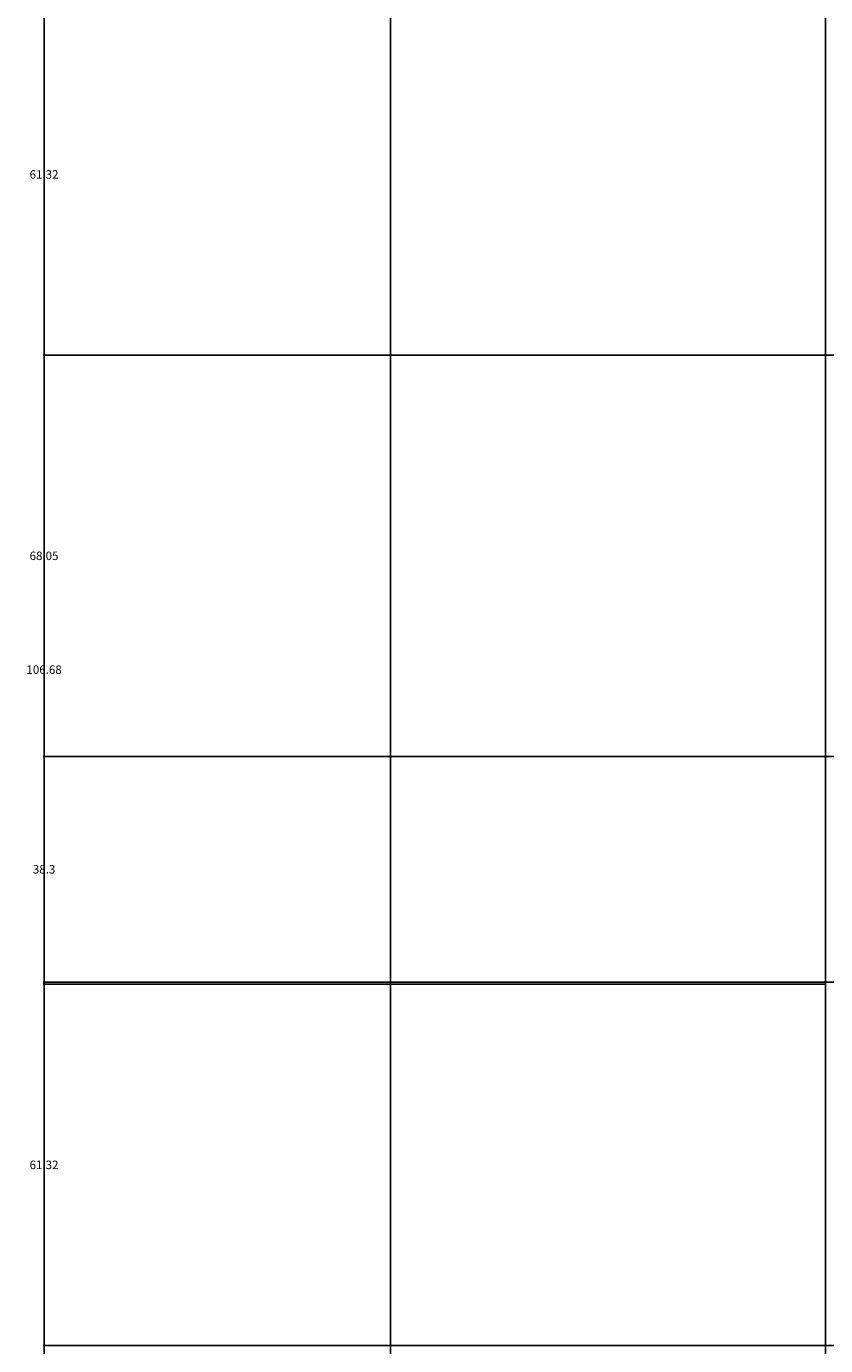
# Model space of a CAD drawing. Units: inches. Extents: x 241 to 943, y 109 to 1396.
# Tile 18 of 34: x 241 to 377, y 842 to 1065. Entities that reach past the tile are written whole.
import ezdxf

# ---------------------------------------------------------------- set-up
doc = ezdxf.new("R2010")
doc.units = ezdxf.units.IN
doc.header["$MEASUREMENT"] = 0
doc.layers.add('A-ANNO-DIMS', color=2, linetype='Continuous', lineweight=18)
doc.styles.get("Standard").update_dxf_attribs({"font": 'arial.ttf'})
doc.dimstyles.get("Standard").update_dxf_attribs({"dimtxt": 1.4375, "dimasz": 0.18, "dimexe": 0.18, "dimexo": 0.0625, "dimgap": 0.09, "dimtad": 0, "dimtih": 1, "dimtoh": 1, "dimdec": 4, "dimzin": 0, "dimdsep": 46, "dimlunit": 4, "dimtxsty": 'Standard', "dimcen": 0.09, "dimadec": 0, "dimazin": 0, "dimtfac": 1, "dimtdec": 4, "dimtofl": 0, "dimtmove": 0, "dimatfit": 3, "dimfxl": 1, "dimtolj": 1, "dimtzin": 0, "dimarcsym": 0})

# ---------------------------------------------------------------- blocks, each defined once
blk = doc.blocks.new('*D5')
at = {"layer": 'A-ANNO-DIMS', "color": 0, "lineweight": -2, "transparency": 16777216}
for p, q in [((303.24, 177.8), (303.24, 1395.05)), ((303.42, 1394.87), (338.18, 1394.87)), ((376.86, 1394.87), (342.09, 1394.87)), ((377.04, 177.76), (377.04, 1395.05))]:
    blk.add_line(p, q, dxfattribs=at)
at = {"layer": 'A-ANNO-DIMS', "color": 0, "transparency": 16777216}
for points in [[(303.42, 1394.9), (303.42, 1394.84), (303.24, 1394.87)], [(376.86, 1394.9), (376.86, 1394.84), (377.04, 1394.87)]]:
    blk.add_solid(points, dxfattribs=at)
at = {"layer": 'Defpoints', "color": 0, "transparency": 16777216}
for p in [(377.04, 1394.87), (303.24, 177.74), (377.04, 177.7)]:
    blk.add_point(p, dxfattribs=at)
at = {"layer": 'A-ANNO-DIMS', "color": 0, "transparency": 16777216, "insert": (340.14, 1394.87), "char_height": 1.438, "attachment_point": 5}
blk.add_mtext('\\A1;73.8', dxfattribs=at)
blk = doc.blocks.new('*D7')
at = {"layer": 'A-ANNO-DIMS', "color": 0, "lineweight": -2, "transparency": 16777216}
for p, q in [((508.24, 1336.12), (244.31, 1336.12)), ((244.49, 1335.94), (244.49, 753.25)), ((244.49, 168.92), (244.49, 751.6)), ((303.17, 168.74), (244.31, 168.74))]:
    blk.add_line(p, q, dxfattribs=at)
at = {"layer": 'A-ANNO-DIMS', "color": 0, "transparency": 16777216}
for points in [[(244.46, 1335.94), (244.52, 1335.94), (244.49, 1336.12)], [(244.46, 168.92), (244.52, 168.92), (244.49, 168.74)]]:
    blk.add_solid(points, dxfattribs=at)
at = {"layer": 'Defpoints', "color": 0, "transparency": 16777216}
for p in [(244.49, 1336.12), (508.31, 1336.12), (303.24, 168.74)]:
    blk.add_point(p, dxfattribs=at)
at = {"layer": 'A-ANNO-DIMS', "color": 0, "transparency": 16777216, "insert": (244.49, 752.43), "char_height": 1.438, "attachment_point": 5}
blk.add_mtext('\\A1;1167.4', dxfattribs=at)
blk = doc.blocks.new('*D8')
at = {"layer": 'A-ANNO-DIMS', "color": 0, "lineweight": -2, "transparency": 16777216}
for p, q in [((377.04, 396.94), (377.04, 1395.05)), ((377.22, 1394.87), (380.96, 1394.87)), ((390.71, 1394.87), (386.97, 1394.87)), ((390.89, 384.24), (390.89, 1395.05))]:
    blk.add_line(p, q, dxfattribs=at)
at = {"layer": 'A-ANNO-DIMS', "color": 0, "transparency": 16777216}
for points in [[(377.22, 1394.9), (377.22, 1394.84), (377.04, 1394.87)], [(390.71, 1394.9), (390.71, 1394.84), (390.89, 1394.87)]]:
    blk.add_solid(points, dxfattribs=at)
at = {"layer": 'Defpoints', "color": 0, "transparency": 16777216}
for p in [(390.89, 1394.87), (377.04, 396.88), (390.89, 384.18)]:
    blk.add_point(p, dxfattribs=at)
at = {"layer": 'A-ANNO-DIMS', "color": 0, "transparency": 16777216, "insert": (383.97, 1394.87), "char_height": 1.438, "attachment_point": 5}
blk.add_mtext('\\A1;13.856', dxfattribs=at)
blk = doc.blocks.new('*D22')
at = {"layer": 'A-ANNO-DIMS', "color": 0, "lineweight": -2, "transparency": 16777216}
for p, q in [((376.98, 841.54), (244.31, 841.54)), ((244.49, 841.36), (244.49, 789.02)), ((244.49, 735.03), (244.49, 787.37)), ((376.98, 734.85), (244.31, 734.85))]:
    blk.add_line(p, q, dxfattribs=at)
at = {"layer": 'A-ANNO-DIMS', "color": 0, "transparency": 16777216}
for points in [[(244.46, 841.36), (244.52, 841.36), (244.49, 841.54)], [(244.46, 735.03), (244.52, 735.03), (244.49, 734.85)]]:
    blk.add_solid(points, dxfattribs=at)
at = {"layer": 'Defpoints', "color": 0, "transparency": 16777216}
for p in [(244.49, 841.54), (377.04, 841.54), (377.04, 734.85)]:
    blk.add_point(p, dxfattribs=at)
at = {"layer": 'A-ANNO-DIMS', "color": 0, "transparency": 16777216, "insert": (244.49, 788.2), "char_height": 1.438, "attachment_point": 5}
blk.add_mtext('\\A1;106.68', dxfattribs=at)
blk = doc.blocks.new('*D23')
at = {"layer": 'A-ANNO-DIMS', "color": 0, "lineweight": -2, "transparency": 16777216}
for p, q in [((376.98, 902.85), (244.31, 902.85)), ((244.49, 902.67), (244.49, 873.02)), ((244.49, 841.72), (244.49, 871.37)), ((376.98, 841.54), (244.31, 841.54))]:
    blk.add_line(p, q, dxfattribs=at)
at = {"layer": 'A-ANNO-DIMS', "color": 0, "transparency": 16777216}
for points in [[(244.46, 902.67), (244.52, 902.67), (244.49, 902.85)], [(244.46, 841.72), (244.52, 841.72), (244.49, 841.54)]]:
    blk.add_solid(points, dxfattribs=at)
at = {"layer": 'Defpoints', "color": 0, "transparency": 16777216}
for p in [(244.49, 902.85), (377.04, 902.85), (377.04, 841.54)]:
    blk.add_point(p, dxfattribs=at)
at = {"layer": 'A-ANNO-DIMS', "color": 0, "transparency": 16777216, "insert": (244.49, 872.2), "char_height": 1.438, "attachment_point": 5}
blk.add_mtext('\\A1;61.32', dxfattribs=at)
blk = doc.blocks.new('*D24')
at = {"layer": 'A-ANNO-DIMS', "color": 0, "lineweight": -2, "transparency": 16777216}
for p, q in [((376.98, 1009.54), (244.31, 1009.54)), ((244.49, 1009.36), (244.49, 957.02)), ((244.49, 903.03), (244.49, 955.37)), ((376.98, 902.85), (244.31, 902.85))]:
    blk.add_line(p, q, dxfattribs=at)
at = {"layer": 'A-ANNO-DIMS', "color": 0, "transparency": 16777216}
for points in [[(244.46, 1009.36), (244.52, 1009.36), (244.49, 1009.54)], [(244.46, 903.03), (244.52, 903.03), (244.49, 902.85)]]:
    blk.add_solid(points, dxfattribs=at)
at = {"layer": 'Defpoints', "color": 0, "transparency": 16777216}
for p in [(244.49, 1009.54), (377.04, 1009.54), (377.04, 902.85)]:
    blk.add_point(p, dxfattribs=at)
at = {"layer": 'A-ANNO-DIMS', "color": 0, "transparency": 16777216, "insert": (244.49, 956.2), "char_height": 1.438, "attachment_point": 5}
blk.add_mtext('\\A1;106.68', dxfattribs=at)
blk = doc.blocks.new('*D25')
at = {"layer": 'A-ANNO-DIMS', "color": 0, "lineweight": -2, "transparency": 16777216}
for p, q in [((376.98, 1070.85), (244.31, 1070.85)), ((244.49, 1070.67), (244.49, 1041.02)), ((244.49, 1009.72), (244.49, 1039.37)), ((376.98, 1009.54), (244.31, 1009.54))]:
    blk.add_line(p, q, dxfattribs=at)
at = {"layer": 'A-ANNO-DIMS', "color": 0, "transparency": 16777216}
for points in [[(244.46, 1070.67), (244.52, 1070.67), (244.49, 1070.85)], [(244.46, 1009.72), (244.52, 1009.72), (244.49, 1009.54)]]:
    blk.add_solid(points, dxfattribs=at)
at = {"layer": 'Defpoints', "color": 0, "transparency": 16777216}
for p in [(244.49, 1070.85), (377.04, 1070.85), (377.04, 1009.54)]:
    blk.add_point(p, dxfattribs=at)
at = {"layer": 'A-ANNO-DIMS', "color": 0, "transparency": 16777216, "insert": (244.49, 1040.2), "char_height": 1.438, "attachment_point": 5}
blk.add_mtext('\\A1;61.32', dxfattribs=at)
blk = doc.blocks.new('*D36')
at = {"layer": 'A-ANNO-DIMS', "color": 0, "lineweight": -2, "transparency": 16777216}
for p, q in [((396.25, 841.54), (244.31, 841.54)), ((244.49, 841.36), (244.49, 808.34)), ((244.49, 773.67), (244.49, 806.69)), ((396.25, 773.49), (244.31, 773.49))]:
    blk.add_line(p, q, dxfattribs=at)
at = {"layer": 'A-ANNO-DIMS', "color": 0, "transparency": 16777216}
for points in [[(244.46, 841.36), (244.52, 841.36), (244.49, 841.54)], [(244.46, 773.67), (244.52, 773.67), (244.49, 773.49)]]:
    blk.add_solid(points, dxfattribs=at)
at = {"layer": 'Defpoints', "color": 0, "transparency": 16777216}
for p in [(244.49, 841.54), (396.31, 841.54), (396.31, 773.49)]:
    blk.add_point(p, dxfattribs=at)
at = {"layer": 'A-ANNO-DIMS', "color": 0, "transparency": 16777216, "insert": (244.49, 807.51), "char_height": 1.438, "attachment_point": 5}
blk.add_mtext('\\A1;68.05', dxfattribs=at)
blk = doc.blocks.new('*D37')
at = {"layer": 'A-ANNO-DIMS', "color": 0, "lineweight": -2, "transparency": 16777216}
for p, q in [((388.98, 941.49), (244.31, 941.49)), ((244.49, 941.31), (244.49, 923.16)), ((244.49, 903.37), (244.49, 921.52)), ((388.98, 903.19), (244.31, 903.19))]:
    blk.add_line(p, q, dxfattribs=at)
at = {"layer": 'A-ANNO-DIMS', "color": 0, "transparency": 16777216}
for points in [[(244.46, 941.31), (244.52, 941.31), (244.49, 941.49)], [(244.46, 903.37), (244.52, 903.37), (244.49, 903.19)]]:
    blk.add_solid(points, dxfattribs=at)
at = {"layer": 'Defpoints', "color": 0, "transparency": 16777216}
for p in [(244.49, 941.49), (389.04, 941.49), (389.04, 903.19)]:
    blk.add_point(p, dxfattribs=at)
at = {"layer": 'A-ANNO-DIMS', "color": 0, "transparency": 16777216, "insert": (244.49, 922.34), "char_height": 1.438, "attachment_point": 5}
blk.add_mtext('\\A1;38.3', dxfattribs=at)
blk = doc.blocks.new('*D38')
at = {"layer": 'A-ANNO-DIMS', "color": 0, "lineweight": -2, "transparency": 16777216}
for p, q in [((396.25, 1009.54), (244.31, 1009.54)), ((244.49, 1009.36), (244.49, 976.34)), ((244.49, 941.67), (244.49, 974.69)), ((396.25, 941.49), (244.31, 941.49))]:
    blk.add_line(p, q, dxfattribs=at)
at = {"layer": 'A-ANNO-DIMS', "color": 0, "transparency": 16777216}
for points in [[(244.46, 1009.36), (244.52, 1009.36), (244.49, 1009.54)], [(244.46, 941.67), (244.52, 941.67), (244.49, 941.49)]]:
    blk.add_solid(points, dxfattribs=at)
at = {"layer": 'Defpoints', "color": 0, "transparency": 16777216}
for p in [(244.49, 1009.54), (396.31, 1009.54), (396.31, 941.49)]:
    blk.add_point(p, dxfattribs=at)
at = {"layer": 'A-ANNO-DIMS', "color": 0, "transparency": 16777216, "insert": (244.49, 975.51), "char_height": 1.438, "attachment_point": 5}
blk.add_mtext('\\A1;68.05', dxfattribs=at)
blk = doc.blocks.new('*D61')
at = {"layer": 'A-ANNO-DIMS', "color": 0, "lineweight": -2, "transparency": 16777216}
for p, q in [((377.04, 400.89), (377.04, 1395.05)), ((377.22, 1394.87), (398.03, 1394.87)), ((423.93, 1394.87), (403.12, 1394.87)), ((424.11, 568.89), (424.11, 1395.05))]:
    blk.add_line(p, q, dxfattribs=at)
at = {"layer": 'A-ANNO-DIMS', "color": 0, "transparency": 16777216}
for points in [[(377.22, 1394.9), (377.22, 1394.84), (377.04, 1394.87)], [(423.93, 1394.9), (423.93, 1394.84), (424.11, 1394.87)]]:
    blk.add_solid(points, dxfattribs=at)
at = {"layer": 'Defpoints', "color": 0, "transparency": 16777216}
for p in [(424.11, 1394.87), (424.11, 568.83), (377.04, 400.83)]:
    blk.add_point(p, dxfattribs=at)
at = {"layer": 'A-ANNO-DIMS', "color": 0, "transparency": 16777216, "insert": (400.57, 1394.87), "char_height": 1.438, "attachment_point": 5}
blk.add_mtext('\\A1;47.07', dxfattribs=at)
blk = doc.blocks.new('*D89')
at = {"layer": 'A-ANNO-DIMS', "color": 0, "lineweight": -2, "transparency": 16777216}
for p, q in [((377.04, 841.6), (377.04, 1395.05)), ((377.22, 1394.87), (494.32, 1394.87)), ((617.58, 1394.87), (500.48, 1394.87)), ((617.76, 841.6), (617.76, 1395.05))]:
    blk.add_line(p, q, dxfattribs=at)
at = {"layer": 'A-ANNO-DIMS', "color": 0, "transparency": 16777216}
for points in [[(377.22, 1394.9), (377.22, 1394.84), (377.04, 1394.87)], [(617.58, 1394.9), (617.58, 1394.84), (617.76, 1394.87)]]:
    blk.add_solid(points, dxfattribs=at)
at = {"layer": 'Defpoints', "color": 0, "transparency": 16777216}
for p in [(617.76, 1394.87), (377.04, 841.54), (617.76, 841.54)]:
    blk.add_point(p, dxfattribs=at)
at = {"layer": 'A-ANNO-DIMS', "color": 0, "transparency": 16777216, "insert": (497.4, 1394.87), "char_height": 1.438, "attachment_point": 5}
blk.add_mtext('\\A1;240.72', dxfattribs=at)
blk = doc.blocks.new('*D91')
at = {"layer": 'A-ANNO-DIMS', "color": 0, "lineweight": -2, "transparency": 16777216}
for p, q in [((377.04, 1070.79), (377.04, 109.81)), ((389.04, 1070.79), (389.04, 109.81)), ((377.22, 109.99), (380.04, 109.99)), ((388.86, 109.99), (386.04, 109.99))]:
    blk.add_line(p, q, dxfattribs=at)
at = {"layer": 'A-ANNO-DIMS', "color": 0, "transparency": 16777216}
for points in [[(377.22, 110.02), (377.22, 109.96), (377.04, 109.99)], [(388.86, 110.02), (388.86, 109.96), (389.04, 109.99)]]:
    blk.add_solid(points, dxfattribs=at)
at = {"layer": 'Defpoints', "color": 0, "transparency": 16777216}
for p in [(377.04, 1070.85), (389.04, 1070.85), (389.04, 109.99)]:
    blk.add_point(p, dxfattribs=at)
at = {"layer": 'A-ANNO-DIMS', "color": 0, "transparency": 16777216, "insert": (383.04, 109.99), "char_height": 1.438, "attachment_point": 5}
blk.add_mtext('\\A1;12.004', dxfattribs=at)

msp = doc.modelspace()

# ---------------------------------------------------------------- dimensions: what is measured, and where the dimension line sits
at = {"layer": 'A-ANNO-DIMS'}
for base, p1, p2, override, picture, middle in [((377.0391, 1394.8654), (303.2358, 177.7407), (377.0391, 177.6977), {"dimdec": 1, "dimlfac": 1, "dimrnd": 0, "dimzin": 0, "dimdsep": 46, "dimlunit": 2}, '*D5', (340.1375, 1394.8654)), ((390.895, 1394.8654), (377.0391, 396.8782), (390.895, 384.1784), {"dimdec": 3, "dimlfac": 1, "dimrnd": 0, "dimzin": 0, "dimdsep": 46, "dimlunit": 2}, '*D8', (383.9671, 1394.8654)), ((424.1086, 1394.8654), (377.0391, 400.8295), (424.1086, 568.8295), {"dimdec": 2, "dimlfac": 1, "dimrnd": 0, "dimzin": 0, "dimdsep": 46, "dimlunit": 2}, '*D61', (400.5739, 1394.8654)), ((617.7594, 1394.8654), (377.0391, 841.5382), (617.7594, 841.5382), {"dimdec": 2, "dimlfac": 1, "dimrnd": 0, "dimzin": 0, "dimdsep": 46, "dimlunit": 2}, '*D89', (497.3993, 1394.8654)), ((389.0429, 109.9907), (377.0391, 1070.8538), (389.0429, 1070.8538), {"dimdec": 3, "dimlfac": 1, "dimrnd": 0, "dimzin": 0, "dimdsep": 46, "dimlunit": 2}, '*D91', (383.041, 109.9907))]:
    dim = msp.add_linear_dim(base=base, p1=p1, p2=p2, dimstyle='Standard', override=override, dxfattribs=at)
    dim.commit()
    dim.dimension.update_dxf_attribs({"geometry": picture, "text_midpoint": middle})
for base, p1, p2, override, picture, middle in [((244.4858, 1336.1154), (303.2358, 168.7407), (508.3064, 1336.1154), {"dimdec": 1, "dimlfac": 1, "dimrnd": 0, "dimzin": 0, "dimdsep": 46, "dimlunit": 2}, '*D7', (244.4858, 752.4281)), ((244.4858, 1070.8538), (377.0391, 1009.5382), (377.0391, 1070.8538), {"dimdec": 2, "dimlfac": 1, "dimrnd": 0, "dimzin": 0, "dimdsep": 46, "dimlunit": 2}, '*D25', (244.4858, 1040.196)), ((244.4858, 1009.5382), (377.0391, 902.8538), (377.0391, 1009.5382), {"dimdec": 2, "dimlfac": 1, "dimrnd": 0, "dimzin": 0, "dimdsep": 46, "dimlunit": 2}, '*D24', (244.4858, 956.196)), ((244.4858, 1009.5382), (396.3125, 941.4916), (396.3125, 1009.5382), {"dimdec": 2, "dimlfac": 1, "dimrnd": 0, "dimzin": 0, "dimdsep": 46, "dimlunit": 2}, '*D38', (244.4858, 975.5149)), ((244.4858, 941.4916), (389.0429, 903.188), (389.0429, 941.4916), {"dimdec": 1, "dimlfac": 1, "dimrnd": 0, "dimzin": 0, "dimdsep": 46, "dimlunit": 2}, '*D37', (244.4858, 922.3398)), ((244.4858, 902.8538), (377.0391, 841.5382), (377.0391, 902.8538), {"dimdec": 2, "dimlfac": 1, "dimrnd": 0, "dimzin": 0, "dimdsep": 46, "dimlunit": 2}, '*D23', (244.4858, 872.196)), ((244.4858, 841.5382), (377.0391, 734.8538), (377.0391, 841.5382), {"dimdec": 2, "dimlfac": 1, "dimrnd": 0, "dimzin": 0, "dimdsep": 46, "dimlunit": 2}, '*D22', (244.4858, 788.196)), ((244.4858, 841.5382), (396.3125, 773.4916), (396.3125, 841.5382), {"dimdec": 2, "dimlfac": 1, "dimrnd": 0, "dimzin": 0, "dimdsep": 46, "dimlunit": 2}, '*D36', (244.4858, 807.5149))]:
    dim = msp.add_linear_dim(base=base, p1=p1, p2=p2, angle=90, dimstyle='Standard', override=override, dxfattribs=at)
    dim.commit()
    dim.dimension.update_dxf_attribs({"geometry": picture, "text_midpoint": middle})

doc.saveas('drawing.dxf')
